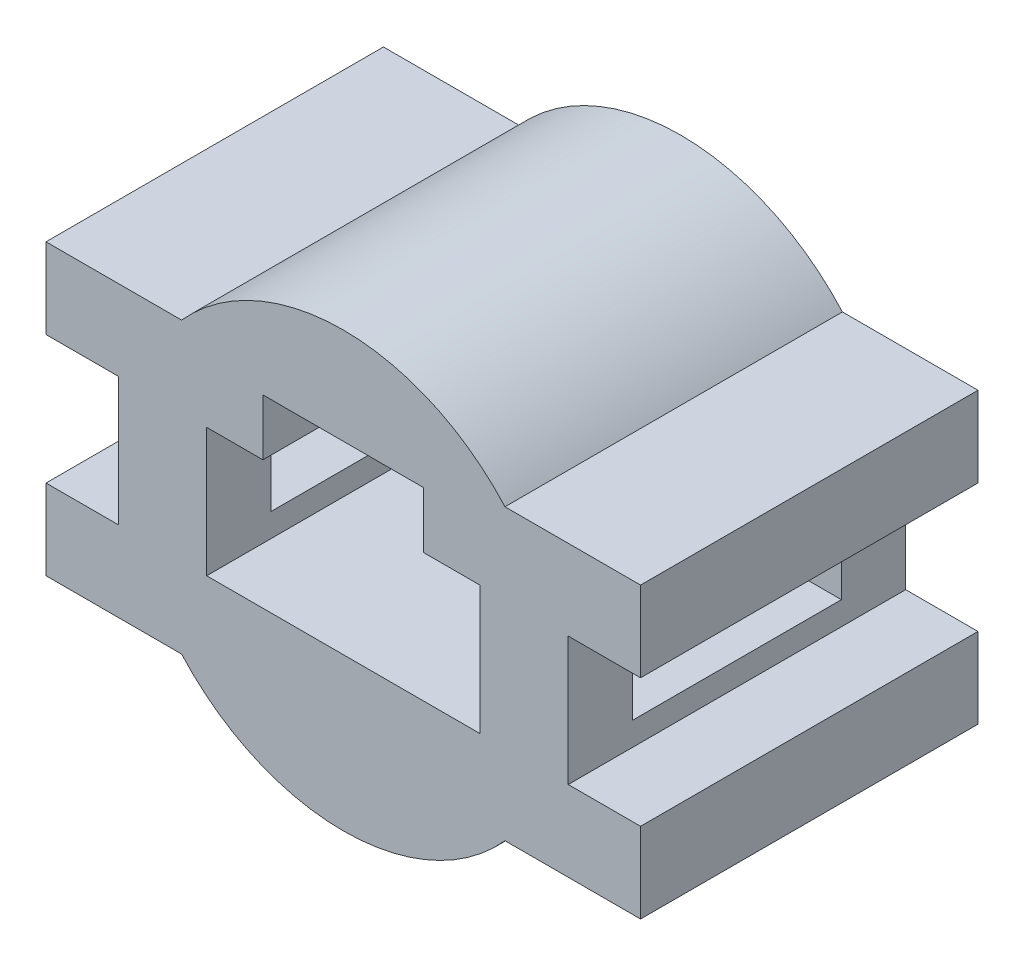
ISO-10303-21;
HEADER;
FILE_DESCRIPTION(('STEP AP214'),'2;1');
FILE_NAME('part.step','',(''),(''),'','','');
FILE_SCHEMA(('AUTOMOTIVE_DESIGN { 1 0 10303 214 1 1 1 1 }'));
ENDSEC;
DATA;
#1=APPLICATION_CONTEXT('core data for automotive mechanical design processes');
#2=APPLICATION_PROTOCOL_DEFINITION('international standard','automotive_design',2000,#1);
#3=PRODUCT_CONTEXT('',#1,'mechanical');
#4=PRODUCT('Part','Part','',(#3));
#5=PRODUCT_RELATED_PRODUCT_CATEGORY('part','',(#4));
#6=PRODUCT_DEFINITION_FORMATION('','',#4);
#7=PRODUCT_DEFINITION_CONTEXT('part definition',#1,'design');
#8=PRODUCT_DEFINITION('design','',#6,#7);
#9=PRODUCT_DEFINITION_SHAPE('','',#8);
#10=(LENGTH_UNIT() NAMED_UNIT(*) SI_UNIT(.MILLI.,.METRE.));
#11=(NAMED_UNIT(*) PLANE_ANGLE_UNIT() SI_UNIT($,.RADIAN.));
#12=(NAMED_UNIT(*) SI_UNIT($,.STERADIAN.) SOLID_ANGLE_UNIT());
#13=UNCERTAINTY_MEASURE_WITH_UNIT(LENGTH_MEASURE(1.E-05),#10,'distance_accuracy_value','');
#14=(GEOMETRIC_REPRESENTATION_CONTEXT(3) GLOBAL_UNCERTAINTY_ASSIGNED_CONTEXT((#13)) GLOBAL_UNIT_ASSIGNED_CONTEXT((#10,
#11,#12)) REPRESENTATION_CONTEXT('',''));
#15=CARTESIAN_POINT('',(0.,0.,0.));
#16=DIRECTION('',(0.,0.,1.));
#17=DIRECTION('',(1.,0.,0.));
#18=AXIS2_PLACEMENT_3D('',#15,#16,#17);
#19=CARTESIAN_POINT('',(0.,0.,-42.));
#20=DIRECTION('',(-1.,0.,0.));
#21=DIRECTION('',(0.,0.,1.));
#22=AXIS2_PLACEMENT_3D('',#19,#20,#21);
#23=PLANE('',#22);
#24=DIRECTION('',(0.,-1.,0.));
#25=VECTOR('',#24,1.);
#26=CARTESIAN_POINT('',(0.,0.,0.));
#27=LINE('',#26,#25);
#28=CARTESIAN_POINT('',(0.,0.,0.));
#29=VERTEX_POINT('',#28);
#30=CARTESIAN_POINT('',(0.,-10.,0.));
#31=VERTEX_POINT('',#30);
#32=EDGE_CURVE('E356',#29,#31,#27,.T.);
#33=ORIENTED_EDGE('',*,*,#32,.F.);
#34=DIRECTION('',(0.,0.,1.));
#35=VECTOR('',#34,1.);
#36=CARTESIAN_POINT('',(0.,0.,-42.));
#37=LINE('',#36,#35);
#38=CARTESIAN_POINT('',(0.,0.,-42.));
#39=VERTEX_POINT('',#38);
#40=EDGE_CURVE('E462',#39,#29,#37,.T.);
#41=ORIENTED_EDGE('',*,*,#40,.F.);
#42=DIRECTION('',(0.,-1.,0.));
#43=VECTOR('',#42,1.);
#44=CARTESIAN_POINT('',(0.,0.,-42.));
#45=LINE('',#44,#43);
#46=CARTESIAN_POINT('',(0.,-10.,-42.));
#47=VERTEX_POINT('',#46);
#48=EDGE_CURVE('E364',#39,#47,#45,.T.);
#49=ORIENTED_EDGE('',*,*,#48,.T.);
#50=DIRECTION('',(0.,0.,1.));
#51=VECTOR('',#50,1.);
#52=CARTESIAN_POINT('',(0.,-10.,-42.));
#53=LINE('',#52,#51);
#54=EDGE_CURVE('E412',#47,#31,#53,.T.);
#55=ORIENTED_EDGE('',*,*,#54,.T.);
#56=EDGE_LOOP('',(#33,#41,#49,#55));
#57=FACE_BOUND('',#56,.T.);
#58=ADVANCED_FACE('F39',(#57),#23,.T.);
#59=CARTESIAN_POINT('',(0.,0.,-42.));
#60=DIRECTION('',(0.,1.,0.));
#61=DIRECTION('',(0.,0.,1.));
#62=AXIS2_PLACEMENT_3D('',#59,#60,#61);
#63=PLANE('',#62);
#64=DIRECTION('',(-1.,0.,0.));
#65=VECTOR('',#64,1.);
#66=CARTESIAN_POINT('',(0.,0.,0.));
#67=LINE('',#66,#65);
#68=CARTESIAN_POINT('',(16.8753882025019,0.,0.));
#69=VERTEX_POINT('',#68);
#70=EDGE_CURVE('E369',#69,#29,#67,.T.);
#71=ORIENTED_EDGE('',*,*,#70,.F.);
#72=DIRECTION('',(0.,0.,1.));
#73=VECTOR('',#72,1.);
#74=CARTESIAN_POINT('',(16.8753882025019,0.,-42.));
#75=LINE('',#74,#73);
#76=CARTESIAN_POINT('',(16.8753882025019,0.,-42.));
#77=VERTEX_POINT('',#76);
#78=EDGE_CURVE('E461',#77,#69,#75,.T.);
#79=ORIENTED_EDGE('',*,*,#78,.F.);
#80=DIRECTION('',(-1.,0.,0.));
#81=VECTOR('',#80,1.);
#82=CARTESIAN_POINT('',(0.,0.,-42.));
#83=LINE('',#82,#81);
#84=EDGE_CURVE('E413',#77,#39,#83,.T.);
#85=ORIENTED_EDGE('',*,*,#84,.T.);
#86=ORIENTED_EDGE('',*,*,#40,.T.);
#87=EDGE_LOOP('',(#71,#79,#85,#86));
#88=FACE_BOUND('',#87,.T.);
#89=ADVANCED_FACE('F513',(#88),#63,.T.);
#90=CARTESIAN_POINT('',(37.,-18.,-42.));
#91=DIRECTION('',(0.,0.,1.));
#92=DIRECTION('',(1.,0.,0.));
#93=AXIS2_PLACEMENT_3D('',#90,#91,#92);
#94=CYLINDRICAL_SURFACE('',#93,27.);
#95=CARTESIAN_POINT('',(37.,-18.,0.));
#96=DIRECTION('',(0.,0.,1.));
#97=DIRECTION('',(1.,0.,0.));
#98=AXIS2_PLACEMENT_3D('',#95,#96,#97);
#99=CIRCLE('',#98,27.);
#100=CARTESIAN_POINT('',(57.1246117974981,0.,0.));
#101=VERTEX_POINT('',#100);
#102=EDGE_CURVE('E457',#101,#69,#99,.T.);
#103=ORIENTED_EDGE('',*,*,#102,.F.);
#104=DIRECTION('',(0.,0.,1.));
#105=VECTOR('',#104,1.);
#106=CARTESIAN_POINT('',(57.1246117974981,0.,-42.));
#107=LINE('',#106,#105);
#108=CARTESIAN_POINT('',(57.1246117974981,0.,-42.));
#109=VERTEX_POINT('',#108);
#110=EDGE_CURVE('E468',#109,#101,#107,.T.);
#111=ORIENTED_EDGE('',*,*,#110,.F.);
#112=CARTESIAN_POINT('',(37.,-18.,-42.));
#113=DIRECTION('',(0.,0.,1.));
#114=DIRECTION('',(1.,0.,0.));
#115=AXIS2_PLACEMENT_3D('',#112,#113,#114);
#116=CIRCLE('',#115,27.);
#117=EDGE_CURVE('E410',#109,#77,#116,.T.);
#118=ORIENTED_EDGE('',*,*,#117,.T.);
#119=ORIENTED_EDGE('',*,*,#78,.T.);
#120=EDGE_LOOP('',(#103,#111,#118,#119));
#121=FACE_BOUND('',#120,.T.);
#122=ADVANCED_FACE('F518',(#121),#94,.T.);
#123=CARTESIAN_POINT('',(57.1246117974981,0.,-42.));
#124=DIRECTION('',(0.,1.,0.));
#125=DIRECTION('',(0.,0.,1.));
#126=AXIS2_PLACEMENT_3D('',#123,#124,#125);
#127=PLANE('',#126);
#128=DIRECTION('',(-1.,0.,0.));
#129=VECTOR('',#128,1.);
#130=CARTESIAN_POINT('',(57.1246117974981,0.,0.));
#131=LINE('',#130,#129);
#132=CARTESIAN_POINT('',(74.,0.,0.));
#133=VERTEX_POINT('',#132);
#134=EDGE_CURVE('E451',#133,#101,#131,.T.);
#135=ORIENTED_EDGE('',*,*,#134,.F.);
#136=DIRECTION('',(0.,0.,1.));
#137=VECTOR('',#136,1.);
#138=CARTESIAN_POINT('',(74.,0.,-42.));
#139=LINE('',#138,#137);
#140=CARTESIAN_POINT('',(74.,0.,-42.));
#141=VERTEX_POINT('',#140);
#142=EDGE_CURVE('E466',#141,#133,#139,.T.);
#143=ORIENTED_EDGE('',*,*,#142,.F.);
#144=DIRECTION('',(-1.,0.,0.));
#145=VECTOR('',#144,1.);
#146=CARTESIAN_POINT('',(57.1246117974981,0.,-42.));
#147=LINE('',#146,#145);
#148=EDGE_CURVE('E403',#141,#109,#147,.T.);
#149=ORIENTED_EDGE('',*,*,#148,.T.);
#150=ORIENTED_EDGE('',*,*,#110,.T.);
#151=EDGE_LOOP('',(#135,#143,#149,#150));
#152=FACE_BOUND('',#151,.T.);
#153=ADVANCED_FACE('F582',(#152),#127,.T.);
#154=CARTESIAN_POINT('',(74.,0.,-42.));
#155=DIRECTION('',(1.,0.,0.));
#156=DIRECTION('',(0.,0.,-1.));
#157=AXIS2_PLACEMENT_3D('',#154,#155,#156);
#158=PLANE('',#157);
#159=DIRECTION('',(0.,1.,0.));
#160=VECTOR('',#159,1.);
#161=CARTESIAN_POINT('',(74.,0.,0.));
#162=LINE('',#161,#160);
#163=CARTESIAN_POINT('',(74.,-10.,0.));
#164=VERTEX_POINT('',#163);
#165=EDGE_CURVE('E448',#164,#133,#162,.T.);
#166=ORIENTED_EDGE('',*,*,#165,.F.);
#167=DIRECTION('',(0.,0.,1.));
#168=VECTOR('',#167,1.);
#169=CARTESIAN_POINT('',(74.,-10.,-42.));
#170=LINE('',#169,#168);
#171=CARTESIAN_POINT('',(74.,-10.,-42.));
#172=VERTEX_POINT('',#171);
#173=EDGE_CURVE('E469',#172,#164,#170,.T.);
#174=ORIENTED_EDGE('',*,*,#173,.F.);
#175=DIRECTION('',(0.,1.,0.));
#176=VECTOR('',#175,1.);
#177=CARTESIAN_POINT('',(74.,0.,-42.));
#178=LINE('',#177,#176);
#179=EDGE_CURVE('E405',#172,#141,#178,.T.);
#180=ORIENTED_EDGE('',*,*,#179,.T.);
#181=ORIENTED_EDGE('',*,*,#142,.T.);
#182=EDGE_LOOP('',(#166,#174,#180,#181));
#183=FACE_BOUND('',#182,.T.);
#184=ADVANCED_FACE('F577',(#183),#158,.T.);
#185=CARTESIAN_POINT('',(74.,-10.,-42.));
#186=DIRECTION('',(0.,-1.,0.));
#187=DIRECTION('',(0.,0.,-1.));
#188=AXIS2_PLACEMENT_3D('',#185,#186,#187);
#189=PLANE('',#188);
#190=DIRECTION('',(1.,0.,0.));
#191=VECTOR('',#190,1.);
#192=CARTESIAN_POINT('',(74.,-10.,0.));
#193=LINE('',#192,#191);
#194=CARTESIAN_POINT('',(65.,-10.,0.));
#195=VERTEX_POINT('',#194);
#196=EDGE_CURVE('E449',#195,#164,#193,.T.);
#197=ORIENTED_EDGE('',*,*,#196,.F.);
#198=DIRECTION('',(0.,0.,1.));
#199=VECTOR('',#198,1.);
#200=CARTESIAN_POINT('',(65.,-10.,-42.));
#201=LINE('',#200,#199);
#202=CARTESIAN_POINT('',(65.,-10.,-42.));
#203=VERTEX_POINT('',#202);
#204=EDGE_CURVE('E472',#203,#195,#201,.T.);
#205=ORIENTED_EDGE('',*,*,#204,.F.);
#206=DIRECTION('',(1.,0.,0.));
#207=VECTOR('',#206,1.);
#208=CARTESIAN_POINT('',(74.,-10.,-42.));
#209=LINE('',#208,#207);
#210=EDGE_CURVE('E397',#203,#172,#209,.T.);
#211=ORIENTED_EDGE('',*,*,#210,.T.);
#212=ORIENTED_EDGE('',*,*,#173,.T.);
#213=EDGE_LOOP('',(#197,#205,#211,#212));
#214=FACE_BOUND('',#213,.T.);
#215=ADVANCED_FACE('F573',(#214),#189,.T.);
#216=CARTESIAN_POINT('',(65.,-10.,-42.));
#217=DIRECTION('',(1.,0.,0.));
#218=DIRECTION('',(0.,0.,-1.));
#219=AXIS2_PLACEMENT_3D('',#216,#217,#218);
#220=PLANE('',#219);
#221=DIRECTION('',(0.,0.,1.));
#222=VECTOR('',#221,1.);
#223=CARTESIAN_POINT('',(65.,-13.075177639069,-42.));
#224=LINE('',#223,#222);
#225=CARTESIAN_POINT('',(65.,-13.075177639069,-34.));
#226=VERTEX_POINT('',#225);
#227=CARTESIAN_POINT('',(65.,-13.075177639069,-8.00000000000001));
#228=VERTEX_POINT('',#227);
#229=EDGE_CURVE('E298',#226,#228,#224,.T.);
#230=ORIENTED_EDGE('',*,*,#229,.F.);
#231=DIRECTION('',(0.,1.,0.));
#232=VECTOR('',#231,1.);
#233=CARTESIAN_POINT('',(65.,-10.,-34.));
#234=LINE('',#233,#232);
#235=CARTESIAN_POINT('',(65.,-23.075177639069,-34.));
#236=VERTEX_POINT('',#235);
#237=EDGE_CURVE('E283',#236,#226,#234,.T.);
#238=ORIENTED_EDGE('',*,*,#237,.F.);
#239=DIRECTION('',(0.,0.,-1.));
#240=VECTOR('',#239,1.);
#241=CARTESIAN_POINT('',(65.,-23.075177639069,-42.));
#242=LINE('',#241,#240);
#243=CARTESIAN_POINT('',(65.,-23.075177639069,-8.));
#244=VERTEX_POINT('',#243);
#245=EDGE_CURVE('E289',#244,#236,#242,.T.);
#246=ORIENTED_EDGE('',*,*,#245,.F.);
#247=DIRECTION('',(0.,-1.,0.));
#248=VECTOR('',#247,1.);
#249=CARTESIAN_POINT('',(65.,-9.99999999999999,-8.00000000000001));
#250=LINE('',#249,#248);
#251=EDGE_CURVE('E293',#228,#244,#250,.T.);
#252=ORIENTED_EDGE('',*,*,#251,.F.);
#253=EDGE_LOOP('',(#230,#238,#246,#252));
#254=FACE_BOUND('',#253,.T.);
#255=DIRECTION('',(0.,1.,0.));
#256=VECTOR('',#255,1.);
#257=CARTESIAN_POINT('',(65.,-10.,0.));
#258=LINE('',#257,#256);
#259=CARTESIAN_POINT('',(65.,-26.,0.));
#260=VERTEX_POINT('',#259);
#261=EDGE_CURVE('E441',#260,#195,#258,.T.);
#262=ORIENTED_EDGE('',*,*,#261,.F.);
#263=DIRECTION('',(0.,0.,1.));
#264=VECTOR('',#263,1.);
#265=CARTESIAN_POINT('',(65.,-26.,-42.));
#266=LINE('',#265,#264);
#267=CARTESIAN_POINT('',(65.,-26.,-42.));
#268=VERTEX_POINT('',#267);
#269=EDGE_CURVE('E475',#268,#260,#266,.T.);
#270=ORIENTED_EDGE('',*,*,#269,.F.);
#271=DIRECTION('',(0.,1.,0.));
#272=VECTOR('',#271,1.);
#273=CARTESIAN_POINT('',(65.,-10.,-42.));
#274=LINE('',#273,#272);
#275=EDGE_CURVE('E398',#268,#203,#274,.T.);
#276=ORIENTED_EDGE('',*,*,#275,.T.);
#277=ORIENTED_EDGE('',*,*,#204,.T.);
#278=EDGE_LOOP('',(#262,#270,#276,#277));
#279=FACE_BOUND('',#278,.T.);
#280=ADVANCED_FACE('F572',(#254,#279),#220,.T.);
#281=CARTESIAN_POINT('',(65.,-26.,-42.));
#282=DIRECTION('',(0.,1.,0.));
#283=DIRECTION('',(0.,0.,1.));
#284=AXIS2_PLACEMENT_3D('',#281,#282,#283);
#285=PLANE('',#284);
#286=DIRECTION('',(-1.,0.,0.));
#287=VECTOR('',#286,1.);
#288=CARTESIAN_POINT('',(65.,-26.,0.));
#289=LINE('',#288,#287);
#290=CARTESIAN_POINT('',(74.,-26.,0.));
#291=VERTEX_POINT('',#290);
#292=EDGE_CURVE('E442',#291,#260,#289,.T.);
#293=ORIENTED_EDGE('',*,*,#292,.F.);
#294=DIRECTION('',(0.,0.,1.));
#295=VECTOR('',#294,1.);
#296=CARTESIAN_POINT('',(74.,-26.,-42.));
#297=LINE('',#296,#295);
#298=CARTESIAN_POINT('',(74.,-26.,-42.));
#299=VERTEX_POINT('',#298);
#300=EDGE_CURVE('E478',#299,#291,#297,.T.);
#301=ORIENTED_EDGE('',*,*,#300,.F.);
#302=DIRECTION('',(-1.,0.,0.));
#303=VECTOR('',#302,1.);
#304=CARTESIAN_POINT('',(65.,-26.,-42.));
#305=LINE('',#304,#303);
#306=EDGE_CURVE('E395',#299,#268,#305,.T.);
#307=ORIENTED_EDGE('',*,*,#306,.T.);
#308=ORIENTED_EDGE('',*,*,#269,.T.);
#309=EDGE_LOOP('',(#293,#301,#307,#308));
#310=FACE_BOUND('',#309,.T.);
#311=ADVANCED_FACE('F570',(#310),#285,.T.);
#312=CARTESIAN_POINT('',(74.,-26.,-42.));
#313=DIRECTION('',(1.,0.,0.));
#314=DIRECTION('',(0.,1.,0.));
#315=AXIS2_PLACEMENT_3D('',#312,#313,#314);
#316=PLANE('',#315);
#317=DIRECTION('',(0.,1.,0.));
#318=VECTOR('',#317,1.);
#319=CARTESIAN_POINT('',(74.,-26.,0.));
#320=LINE('',#319,#318);
#321=CARTESIAN_POINT('',(74.,-36.,0.));
#322=VERTEX_POINT('',#321);
#323=EDGE_CURVE('E437',#322,#291,#320,.T.);
#324=ORIENTED_EDGE('',*,*,#323,.F.);
#325=DIRECTION('',(0.,0.,1.));
#326=VECTOR('',#325,1.);
#327=CARTESIAN_POINT('',(74.,-36.,-42.));
#328=LINE('',#327,#326);
#329=CARTESIAN_POINT('',(74.,-36.,-42.));
#330=VERTEX_POINT('',#329);
#331=EDGE_CURVE('E476',#330,#322,#328,.T.);
#332=ORIENTED_EDGE('',*,*,#331,.F.);
#333=DIRECTION('',(0.,1.,0.));
#334=VECTOR('',#333,1.);
#335=CARTESIAN_POINT('',(74.,-26.,-42.));
#336=LINE('',#335,#334);
#337=EDGE_CURVE('E388',#330,#299,#336,.T.);
#338=ORIENTED_EDGE('',*,*,#337,.T.);
#339=ORIENTED_EDGE('',*,*,#300,.T.);
#340=EDGE_LOOP('',(#324,#332,#338,#339));
#341=FACE_BOUND('',#340,.T.);
#342=ADVANCED_FACE('F561',(#341),#316,.T.);
#343=CARTESIAN_POINT('',(74.,-36.,-42.));
#344=DIRECTION('',(0.,-1.,0.));
#345=DIRECTION('',(0.,0.,-1.));
#346=AXIS2_PLACEMENT_3D('',#343,#344,#345);
#347=PLANE('',#346);
#348=DIRECTION('',(1.,0.,0.));
#349=VECTOR('',#348,1.);
#350=CARTESIAN_POINT('',(74.,-36.,0.));
#351=LINE('',#350,#349);
#352=CARTESIAN_POINT('',(57.1246117974981,-36.,0.));
#353=VERTEX_POINT('',#352);
#354=EDGE_CURVE('E434',#353,#322,#351,.T.);
#355=ORIENTED_EDGE('',*,*,#354,.F.);
#356=DIRECTION('',(0.,0.,1.));
#357=VECTOR('',#356,1.);
#358=CARTESIAN_POINT('',(57.1246117974981,-36.,-42.));
#359=LINE('',#358,#357);
#360=CARTESIAN_POINT('',(57.1246117974981,-36.,-42.));
#361=VERTEX_POINT('',#360);
#362=EDGE_CURVE('E477',#361,#353,#359,.T.);
#363=ORIENTED_EDGE('',*,*,#362,.F.);
#364=DIRECTION('',(1.,0.,0.));
#365=VECTOR('',#364,1.);
#366=CARTESIAN_POINT('',(74.,-36.,-42.));
#367=LINE('',#366,#365);
#368=EDGE_CURVE('E390',#361,#330,#367,.T.);
#369=ORIENTED_EDGE('',*,*,#368,.T.);
#370=ORIENTED_EDGE('',*,*,#331,.T.);
#371=EDGE_LOOP('',(#355,#363,#369,#370));
#372=FACE_BOUND('',#371,.T.);
#373=ADVANCED_FACE('F556',(#372),#347,.T.);
#374=CARTESIAN_POINT('',(37.,-18.,-42.));
#375=DIRECTION('',(0.,0.,1.));
#376=DIRECTION('',(1.,0.,0.));
#377=AXIS2_PLACEMENT_3D('',#374,#375,#376);
#378=CYLINDRICAL_SURFACE('',#377,27.);
#379=CARTESIAN_POINT('',(37.,-18.,0.));
#380=DIRECTION('',(0.,0.,1.));
#381=DIRECTION('',(1.,0.,0.));
#382=AXIS2_PLACEMENT_3D('',#379,#380,#381);
#383=CIRCLE('',#382,27.);
#384=CARTESIAN_POINT('',(16.8753882025019,-36.,0.));
#385=VERTEX_POINT('',#384);
#386=EDGE_CURVE('E435',#385,#353,#383,.T.);
#387=ORIENTED_EDGE('',*,*,#386,.F.);
#388=DIRECTION('',(0.,0.,1.));
#389=VECTOR('',#388,1.);
#390=CARTESIAN_POINT('',(16.8753882025019,-36.,-42.));
#391=LINE('',#390,#389);
#392=CARTESIAN_POINT('',(16.8753882025019,-36.,-42.));
#393=VERTEX_POINT('',#392);
#394=EDGE_CURVE('E485',#393,#385,#391,.T.);
#395=ORIENTED_EDGE('',*,*,#394,.F.);
#396=CARTESIAN_POINT('',(37.,-18.,-42.));
#397=DIRECTION('',(0.,0.,1.));
#398=DIRECTION('',(1.,0.,0.));
#399=AXIS2_PLACEMENT_3D('',#396,#397,#398);
#400=CIRCLE('',#399,27.);
#401=EDGE_CURVE('E383',#393,#361,#400,.T.);
#402=ORIENTED_EDGE('',*,*,#401,.T.);
#403=ORIENTED_EDGE('',*,*,#362,.T.);
#404=EDGE_LOOP('',(#387,#395,#402,#403));
#405=FACE_BOUND('',#404,.T.);
#406=ADVANCED_FACE('F553',(#405),#378,.T.);
#407=CARTESIAN_POINT('',(16.8753882025019,-36.,-42.));
#408=DIRECTION('',(0.,-1.,0.));
#409=DIRECTION('',(0.,0.,-1.));
#410=AXIS2_PLACEMENT_3D('',#407,#408,#409);
#411=PLANE('',#410);
#412=DIRECTION('',(1.,0.,0.));
#413=VECTOR('',#412,1.);
#414=CARTESIAN_POINT('',(16.8753882025019,-36.,0.));
#415=LINE('',#414,#413);
#416=CARTESIAN_POINT('',(0.,-36.,0.));
#417=VERTEX_POINT('',#416);
#418=EDGE_CURVE('E427',#417,#385,#415,.T.);
#419=ORIENTED_EDGE('',*,*,#418,.F.);
#420=DIRECTION('',(0.,0.,1.));
#421=VECTOR('',#420,1.);
#422=CARTESIAN_POINT('',(0.,-36.,-42.));
#423=LINE('',#422,#421);
#424=CARTESIAN_POINT('',(0.,-36.,-42.));
#425=VERTEX_POINT('',#424);
#426=EDGE_CURVE('E482',#425,#417,#423,.T.);
#427=ORIENTED_EDGE('',*,*,#426,.F.);
#428=DIRECTION('',(1.,0.,0.));
#429=VECTOR('',#428,1.);
#430=CARTESIAN_POINT('',(16.8753882025019,-36.,-42.));
#431=LINE('',#430,#429);
#432=EDGE_CURVE('E381',#425,#393,#431,.T.);
#433=ORIENTED_EDGE('',*,*,#432,.T.);
#434=ORIENTED_EDGE('',*,*,#394,.T.);
#435=EDGE_LOOP('',(#419,#427,#433,#434));
#436=FACE_BOUND('',#435,.T.);
#437=ADVANCED_FACE('F552',(#436),#411,.T.);
#438=CARTESIAN_POINT('',(0.,-26.,-42.));
#439=DIRECTION('',(-1.,0.,0.));
#440=DIRECTION('',(0.,-1.,0.));
#441=AXIS2_PLACEMENT_3D('',#438,#439,#440);
#442=PLANE('',#441);
#443=DIRECTION('',(0.,-1.,0.));
#444=VECTOR('',#443,1.);
#445=CARTESIAN_POINT('',(0.,-26.,0.));
#446=LINE('',#445,#444);
#447=CARTESIAN_POINT('',(0.,-26.,0.));
#448=VERTEX_POINT('',#447);
#449=EDGE_CURVE('E426',#448,#417,#446,.T.);
#450=ORIENTED_EDGE('',*,*,#449,.F.);
#451=DIRECTION('',(0.,0.,1.));
#452=VECTOR('',#451,1.);
#453=CARTESIAN_POINT('',(0.,-26.,-42.));
#454=LINE('',#453,#452);
#455=CARTESIAN_POINT('',(0.,-26.,-42.));
#456=VERTEX_POINT('',#455);
#457=EDGE_CURVE('E486',#456,#448,#454,.T.);
#458=ORIENTED_EDGE('',*,*,#457,.F.);
#459=DIRECTION('',(0.,-1.,0.));
#460=VECTOR('',#459,1.);
#461=CARTESIAN_POINT('',(0.,-26.,-42.));
#462=LINE('',#461,#460);
#463=EDGE_CURVE('E378',#456,#425,#462,.T.);
#464=ORIENTED_EDGE('',*,*,#463,.T.);
#465=ORIENTED_EDGE('',*,*,#426,.T.);
#466=EDGE_LOOP('',(#450,#458,#464,#465));
#467=FACE_BOUND('',#466,.T.);
#468=ADVANCED_FACE('F550',(#467),#442,.T.);
#469=CARTESIAN_POINT('',(8.99999999999999,-26.,-42.));
#470=DIRECTION('',(0.,1.,0.));
#471=DIRECTION('',(0.,0.,1.));
#472=AXIS2_PLACEMENT_3D('',#469,#470,#471);
#473=PLANE('',#472);
#474=DIRECTION('',(-1.,0.,0.));
#475=VECTOR('',#474,1.);
#476=CARTESIAN_POINT('',(8.99999999999999,-26.,0.));
#477=LINE('',#476,#475);
#478=CARTESIAN_POINT('',(8.99999999999999,-26.,0.));
#479=VERTEX_POINT('',#478);
#480=EDGE_CURVE('E421',#479,#448,#477,.T.);
#481=ORIENTED_EDGE('',*,*,#480,.F.);
#482=DIRECTION('',(0.,0.,1.));
#483=VECTOR('',#482,1.);
#484=CARTESIAN_POINT('',(8.99999999999999,-26.,-42.));
#485=LINE('',#484,#483);
#486=CARTESIAN_POINT('',(8.99999999999999,-26.,-42.));
#487=VERTEX_POINT('',#486);
#488=EDGE_CURVE('E488',#487,#479,#485,.T.);
#489=ORIENTED_EDGE('',*,*,#488,.F.);
#490=DIRECTION('',(-1.,0.,0.));
#491=VECTOR('',#490,1.);
#492=CARTESIAN_POINT('',(8.99999999999999,-26.,-42.));
#493=LINE('',#492,#491);
#494=EDGE_CURVE('E374',#487,#456,#493,.T.);
#495=ORIENTED_EDGE('',*,*,#494,.T.);
#496=ORIENTED_EDGE('',*,*,#457,.T.);
#497=EDGE_LOOP('',(#481,#489,#495,#496));
#498=FACE_BOUND('',#497,.T.);
#499=ADVANCED_FACE('F543',(#498),#473,.T.);
#500=CARTESIAN_POINT('',(8.99999999999999,-10.,-42.));
#501=DIRECTION('',(-1.,0.,0.));
#502=DIRECTION('',(0.,-1.,0.));
#503=AXIS2_PLACEMENT_3D('',#500,#501,#502);
#504=PLANE('',#503);
#505=DIRECTION('',(0.,0.,-1.));
#506=VECTOR('',#505,1.);
#507=CARTESIAN_POINT('',(8.99999999999999,-13.075177639069,-34.));
#508=LINE('',#507,#506);
#509=CARTESIAN_POINT('',(8.99999999999999,-13.075177639069,-8.00000000000001));
#510=VERTEX_POINT('',#509);
#511=CARTESIAN_POINT('',(8.99999999999999,-13.075177639069,-34.));
#512=VERTEX_POINT('',#511);
#513=EDGE_CURVE('E62',#510,#512,#508,.T.);
#514=ORIENTED_EDGE('',*,*,#513,.F.);
#515=DIRECTION('',(0.,1.,0.));
#516=VECTOR('',#515,1.);
#517=CARTESIAN_POINT('',(8.99999999999999,-13.075177639069,-8.00000000000001));
#518=LINE('',#517,#516);
#519=CARTESIAN_POINT('',(8.99999999999999,-23.075177639069,-8.));
#520=VERTEX_POINT('',#519);
#521=EDGE_CURVE('E269',#520,#510,#518,.T.);
#522=ORIENTED_EDGE('',*,*,#521,.F.);
#523=DIRECTION('',(0.,0.,1.));
#524=VECTOR('',#523,1.);
#525=CARTESIAN_POINT('',(8.99999999999999,-23.075177639069,-8.));
#526=LINE('',#525,#524);
#527=CARTESIAN_POINT('',(8.99999999999999,-23.075177639069,-34.));
#528=VERTEX_POINT('',#527);
#529=EDGE_CURVE('E251',#528,#520,#526,.T.);
#530=ORIENTED_EDGE('',*,*,#529,.F.);
#531=DIRECTION('',(0.,-1.,0.));
#532=VECTOR('',#531,1.);
#533=CARTESIAN_POINT('',(8.99999999999999,-23.075177639069,-34.));
#534=LINE('',#533,#532);
#535=EDGE_CURVE('E265',#512,#528,#534,.T.);
#536=ORIENTED_EDGE('',*,*,#535,.F.);
#537=EDGE_LOOP('',(#514,#522,#530,#536));
#538=FACE_BOUND('',#537,.T.);
#539=DIRECTION('',(0.,-1.,0.));
#540=VECTOR('',#539,1.);
#541=CARTESIAN_POINT('',(8.99999999999999,-10.,0.));
#542=LINE('',#541,#540);
#543=CARTESIAN_POINT('',(8.99999999999999,-10.,0.));
#544=VERTEX_POINT('',#543);
#545=EDGE_CURVE('E419',#544,#479,#542,.T.);
#546=ORIENTED_EDGE('',*,*,#545,.F.);
#547=DIRECTION('',(0.,0.,1.));
#548=VECTOR('',#547,1.);
#549=CARTESIAN_POINT('',(8.99999999999999,-10.,-42.));
#550=LINE('',#549,#548);
#551=CARTESIAN_POINT('',(8.99999999999999,-10.,-42.));
#552=VERTEX_POINT('',#551);
#553=EDGE_CURVE('E489',#552,#544,#550,.T.);
#554=ORIENTED_EDGE('',*,*,#553,.F.);
#555=DIRECTION('',(0.,-1.,0.));
#556=VECTOR('',#555,1.);
#557=CARTESIAN_POINT('',(8.99999999999999,-10.,-42.));
#558=LINE('',#557,#556);
#559=EDGE_CURVE('E375',#552,#487,#558,.T.);
#560=ORIENTED_EDGE('',*,*,#559,.T.);
#561=ORIENTED_EDGE('',*,*,#488,.T.);
#562=EDGE_LOOP('',(#546,#554,#560,#561));
#563=FACE_BOUND('',#562,.T.);
#564=ADVANCED_FACE('F270',(#538,#563),#504,.T.);
#565=CARTESIAN_POINT('',(0.,-10.,-42.));
#566=DIRECTION('',(0.,-1.,0.));
#567=DIRECTION('',(0.,0.,-1.));
#568=AXIS2_PLACEMENT_3D('',#565,#566,#567);
#569=PLANE('',#568);
#570=DIRECTION('',(1.,0.,0.));
#571=VECTOR('',#570,1.);
#572=CARTESIAN_POINT('',(0.,-10.,0.));
#573=LINE('',#572,#571);
#574=EDGE_CURVE('E417',#31,#544,#573,.T.);
#575=ORIENTED_EDGE('',*,*,#574,.F.);
#576=ORIENTED_EDGE('',*,*,#54,.F.);
#577=DIRECTION('',(1.,0.,0.));
#578=VECTOR('',#577,1.);
#579=CARTESIAN_POINT('',(0.,-10.,-42.));
#580=LINE('',#579,#578);
#581=EDGE_CURVE('E366',#47,#552,#580,.T.);
#582=ORIENTED_EDGE('',*,*,#581,.T.);
#583=ORIENTED_EDGE('',*,*,#553,.T.);
#584=EDGE_LOOP('',(#575,#576,#582,#583));
#585=FACE_BOUND('',#584,.T.);
#586=ADVANCED_FACE('F537',(#585),#569,.T.);
#587=CARTESIAN_POINT('',(37.,-18.,-42.));
#588=DIRECTION('',(0.,0.,1.));
#589=DIRECTION('',(1.,0.,0.));
#590=AXIS2_PLACEMENT_3D('',#587,#588,#589);
#591=PLANE('',#590);
#592=DIRECTION('',(0.,1.,0.));
#593=VECTOR('',#592,1.);
#594=CARTESIAN_POINT('',(54.,-10.,-42.));
#595=LINE('',#594,#593);
#596=CARTESIAN_POINT('',(54.,-26.,-42.));
#597=VERTEX_POINT('',#596);
#598=CARTESIAN_POINT('',(54.,-10.,-42.));
#599=VERTEX_POINT('',#598);
#600=EDGE_CURVE('E343',#597,#599,#595,.T.);
#601=ORIENTED_EDGE('',*,*,#600,.T.);
#602=DIRECTION('',(-1.,0.,0.));
#603=VECTOR('',#602,1.);
#604=CARTESIAN_POINT('',(27.,-10.,-42.));
#605=LINE('',#604,#603);
#606=CARTESIAN_POINT('',(20.,-10.,-42.));
#607=VERTEX_POINT('',#606);
#608=EDGE_CURVE('E332',#599,#607,#605,.T.);
#609=ORIENTED_EDGE('',*,*,#608,.T.);
#610=DIRECTION('',(0.,-1.,0.));
#611=VECTOR('',#610,1.);
#612=CARTESIAN_POINT('',(20.,-26.,-42.));
#613=LINE('',#612,#611);
#614=CARTESIAN_POINT('',(20.,-26.,-42.));
#615=VERTEX_POINT('',#614);
#616=EDGE_CURVE('E331',#607,#615,#613,.T.);
#617=ORIENTED_EDGE('',*,*,#616,.T.);
#618=DIRECTION('',(1.,0.,0.));
#619=VECTOR('',#618,1.);
#620=CARTESIAN_POINT('',(54.,-26.,-42.));
#621=LINE('',#620,#619);
#622=EDGE_CURVE('E340',#615,#597,#621,.T.);
#623=ORIENTED_EDGE('',*,*,#622,.T.);
#624=EDGE_LOOP('',(#601,#609,#617,#623));
#625=FACE_BOUND('',#624,.T.);
#626=ORIENTED_EDGE('',*,*,#48,.F.);
#627=ORIENTED_EDGE('',*,*,#84,.F.);
#628=ORIENTED_EDGE('',*,*,#117,.F.);
#629=ORIENTED_EDGE('',*,*,#148,.F.);
#630=ORIENTED_EDGE('',*,*,#179,.F.);
#631=ORIENTED_EDGE('',*,*,#210,.F.);
#632=ORIENTED_EDGE('',*,*,#275,.F.);
#633=ORIENTED_EDGE('',*,*,#306,.F.);
#634=ORIENTED_EDGE('',*,*,#337,.F.);
#635=ORIENTED_EDGE('',*,*,#368,.F.);
#636=ORIENTED_EDGE('',*,*,#401,.F.);
#637=ORIENTED_EDGE('',*,*,#432,.F.);
#638=ORIENTED_EDGE('',*,*,#463,.F.);
#639=ORIENTED_EDGE('',*,*,#494,.F.);
#640=ORIENTED_EDGE('',*,*,#559,.F.);
#641=ORIENTED_EDGE('',*,*,#581,.F.);
#642=EDGE_LOOP('',(#626,#627,#628,#629,#630,#631,#632,#633,#634,#635,#636,#637,#638,#639,#640,#641));
#643=FACE_BOUND('',#642,.T.);
#644=ADVANCED_FACE('F531',(#625,#643),#591,.F.);
#645=CARTESIAN_POINT('',(37.,-18.,0.));
#646=DIRECTION('',(0.,0.,1.));
#647=DIRECTION('',(1.,0.,0.));
#648=AXIS2_PLACEMENT_3D('',#645,#646,#647);
#649=PLANE('',#648);
#650=DIRECTION('',(0.,-1.,0.));
#651=VECTOR('',#650,1.);
#652=CARTESIAN_POINT('',(27.,-10.,0.));
#653=LINE('',#652,#651);
#654=CARTESIAN_POINT('',(27.,-3.00000000000001,0.));
#655=VERTEX_POINT('',#654);
#656=CARTESIAN_POINT('',(27.,-10.,0.));
#657=VERTEX_POINT('',#656);
#658=EDGE_CURVE('E307',#655,#657,#653,.T.);
#659=ORIENTED_EDGE('',*,*,#658,.F.);
#660=DIRECTION('',(-1.,0.,0.));
#661=VECTOR('',#660,1.);
#662=CARTESIAN_POINT('',(27.,-3.00000000000001,0.));
#663=LINE('',#662,#661);
#664=CARTESIAN_POINT('',(47.,-3.00000000000001,0.));
#665=VERTEX_POINT('',#664);
#666=EDGE_CURVE('E318',#665,#655,#663,.T.);
#667=ORIENTED_EDGE('',*,*,#666,.F.);
#668=DIRECTION('',(0.,1.,0.));
#669=VECTOR('',#668,1.);
#670=CARTESIAN_POINT('',(47.,-3.00000000000001,0.));
#671=LINE('',#670,#669);
#672=CARTESIAN_POINT('',(47.,-10.,0.));
#673=VERTEX_POINT('',#672);
#674=EDGE_CURVE('E305',#673,#665,#671,.T.);
#675=ORIENTED_EDGE('',*,*,#674,.F.);
#676=DIRECTION('',(-1.,0.,0.));
#677=VECTOR('',#676,1.);
#678=CARTESIAN_POINT('',(47.,-10.,0.));
#679=LINE('',#678,#677);
#680=CARTESIAN_POINT('',(54.,-10.,0.));
#681=VERTEX_POINT('',#680);
#682=EDGE_CURVE('E333',#681,#673,#679,.T.);
#683=ORIENTED_EDGE('',*,*,#682,.F.);
#684=DIRECTION('',(0.,1.,0.));
#685=VECTOR('',#684,1.);
#686=CARTESIAN_POINT('',(54.,-10.,0.));
#687=LINE('',#686,#685);
#688=CARTESIAN_POINT('',(54.,-26.,0.));
#689=VERTEX_POINT('',#688);
#690=EDGE_CURVE('E348',#689,#681,#687,.T.);
#691=ORIENTED_EDGE('',*,*,#690,.F.);
#692=DIRECTION('',(1.,0.,0.));
#693=VECTOR('',#692,1.);
#694=CARTESIAN_POINT('',(54.,-26.,0.));
#695=LINE('',#694,#693);
#696=CARTESIAN_POINT('',(20.,-26.,0.));
#697=VERTEX_POINT('',#696);
#698=EDGE_CURVE('E350',#697,#689,#695,.T.);
#699=ORIENTED_EDGE('',*,*,#698,.F.);
#700=DIRECTION('',(0.,-1.,0.));
#701=VECTOR('',#700,1.);
#702=CARTESIAN_POINT('',(20.,-26.,0.));
#703=LINE('',#702,#701);
#704=CARTESIAN_POINT('',(20.,-10.,0.));
#705=VERTEX_POINT('',#704);
#706=EDGE_CURVE('E324',#705,#697,#703,.T.);
#707=ORIENTED_EDGE('',*,*,#706,.F.);
#708=EDGE_CURVE('E355',#657,#705,#679,.T.);
#709=ORIENTED_EDGE('',*,*,#708,.F.);
#710=EDGE_LOOP('',(#659,#667,#675,#683,#691,#699,#707,#709));
#711=FACE_BOUND('',#710,.T.);
#712=ORIENTED_EDGE('',*,*,#32,.T.);
#713=ORIENTED_EDGE('',*,*,#574,.T.);
#714=ORIENTED_EDGE('',*,*,#545,.T.);
#715=ORIENTED_EDGE('',*,*,#480,.T.);
#716=ORIENTED_EDGE('',*,*,#449,.T.);
#717=ORIENTED_EDGE('',*,*,#418,.T.);
#718=ORIENTED_EDGE('',*,*,#386,.T.);
#719=ORIENTED_EDGE('',*,*,#354,.T.);
#720=ORIENTED_EDGE('',*,*,#323,.T.);
#721=ORIENTED_EDGE('',*,*,#292,.T.);
#722=ORIENTED_EDGE('',*,*,#261,.T.);
#723=ORIENTED_EDGE('',*,*,#196,.T.);
#724=ORIENTED_EDGE('',*,*,#165,.T.);
#725=ORIENTED_EDGE('',*,*,#134,.T.);
#726=ORIENTED_EDGE('',*,*,#102,.T.);
#727=ORIENTED_EDGE('',*,*,#70,.T.);
#728=EDGE_LOOP('',(#712,#713,#714,#715,#716,#717,#718,#719,#720,#721,#722,#723,#724,#725,#726,#727));
#729=FACE_BOUND('',#728,.T.);
#730=ADVANCED_FACE('F526',(#711,#729),#649,.T.);
#731=CARTESIAN_POINT('',(47.,-10.,-42.));
#732=DIRECTION('',(0.,1.,0.));
#733=DIRECTION('',(-1.,0.,0.));
#734=AXIS2_PLACEMENT_3D('',#731,#732,#733);
#735=PLANE('',#734);
#736=DIRECTION('',(1.,0.,0.));
#737=VECTOR('',#736,1.);
#738=CARTESIAN_POINT('',(27.,-10.,-10.));
#739=LINE('',#738,#737);
#740=CARTESIAN_POINT('',(27.,-9.99999999999999,-10.));
#741=VERTEX_POINT('',#740);
#742=CARTESIAN_POINT('',(47.,-10.,-10.));
#743=VERTEX_POINT('',#742);
#744=EDGE_CURVE('E301',#741,#743,#739,.T.);
#745=ORIENTED_EDGE('',*,*,#744,.F.);
#746=DIRECTION('',(0.,0.,1.));
#747=VECTOR('',#746,1.);
#748=CARTESIAN_POINT('',(27.,-10.,-10.));
#749=LINE('',#748,#747);
#750=EDGE_CURVE('E325',#741,#657,#749,.T.);
#751=ORIENTED_EDGE('',*,*,#750,.T.);
#752=ORIENTED_EDGE('',*,*,#708,.T.);
#753=DIRECTION('',(0.,0.,1.));
#754=VECTOR('',#753,1.);
#755=CARTESIAN_POINT('',(20.,-10.,-42.));
#756=LINE('',#755,#754);
#757=EDGE_CURVE('E342',#607,#705,#756,.T.);
#758=ORIENTED_EDGE('',*,*,#757,.F.);
#759=ORIENTED_EDGE('',*,*,#608,.F.);
#760=DIRECTION('',(0.,0.,1.));
#761=VECTOR('',#760,1.);
#762=CARTESIAN_POINT('',(54.,-10.,-42.));
#763=LINE('',#762,#761);
#764=EDGE_CURVE('E358',#599,#681,#763,.T.);
#765=ORIENTED_EDGE('',*,*,#764,.T.);
#766=ORIENTED_EDGE('',*,*,#682,.T.);
#767=DIRECTION('',(0.,0.,1.));
#768=VECTOR('',#767,1.);
#769=CARTESIAN_POINT('',(47.,-10.,-10.));
#770=LINE('',#769,#768);
#771=EDGE_CURVE('E312',#743,#673,#770,.T.);
#772=ORIENTED_EDGE('',*,*,#771,.F.);
#773=EDGE_LOOP('',(#745,#751,#752,#758,#759,#765,#766,#772));
#774=FACE_BOUND('',#773,.T.);
#775=ADVANCED_FACE('F624',(#774),#735,.F.);
#776=CARTESIAN_POINT('',(54.,-10.,-42.));
#777=DIRECTION('',(1.,0.,0.));
#778=DIRECTION('',(0.,0.,-1.));
#779=AXIS2_PLACEMENT_3D('',#776,#777,#778);
#780=PLANE('',#779);
#781=DIRECTION('',(0.,1.,0.));
#782=VECTOR('',#781,1.);
#783=CARTESIAN_POINT('',(54.,-10.,-34.));
#784=LINE('',#783,#782);
#785=CARTESIAN_POINT('',(54.,-23.075177639069,-34.));
#786=VERTEX_POINT('',#785);
#787=CARTESIAN_POINT('',(54.,-13.075177639069,-34.));
#788=VERTEX_POINT('',#787);
#789=EDGE_CURVE('E284',#786,#788,#784,.T.);
#790=ORIENTED_EDGE('',*,*,#789,.T.);
#791=DIRECTION('',(0.,0.,1.));
#792=VECTOR('',#791,1.);
#793=CARTESIAN_POINT('',(54.,-13.075177639069,-42.));
#794=LINE('',#793,#792);
#795=CARTESIAN_POINT('',(54.,-13.075177639069,-8.00000000000001));
#796=VERTEX_POINT('',#795);
#797=EDGE_CURVE('E299',#788,#796,#794,.T.);
#798=ORIENTED_EDGE('',*,*,#797,.T.);
#799=DIRECTION('',(0.,-1.,0.));
#800=VECTOR('',#799,1.);
#801=CARTESIAN_POINT('',(54.,-9.99999999999999,-8.00000000000001));
#802=LINE('',#801,#800);
#803=CARTESIAN_POINT('',(54.,-23.075177639069,-8.));
#804=VERTEX_POINT('',#803);
#805=EDGE_CURVE('E295',#796,#804,#802,.T.);
#806=ORIENTED_EDGE('',*,*,#805,.T.);
#807=DIRECTION('',(0.,0.,-1.));
#808=VECTOR('',#807,1.);
#809=CARTESIAN_POINT('',(54.,-23.075177639069,-42.));
#810=LINE('',#809,#808);
#811=EDGE_CURVE('E290',#804,#786,#810,.T.);
#812=ORIENTED_EDGE('',*,*,#811,.T.);
#813=EDGE_LOOP('',(#790,#798,#806,#812));
#814=FACE_BOUND('',#813,.T.);
#815=ORIENTED_EDGE('',*,*,#690,.T.);
#816=ORIENTED_EDGE('',*,*,#764,.F.);
#817=ORIENTED_EDGE('',*,*,#600,.F.);
#818=DIRECTION('',(0.,0.,1.));
#819=VECTOR('',#818,1.);
#820=CARTESIAN_POINT('',(54.,-26.,-42.));
#821=LINE('',#820,#819);
#822=EDGE_CURVE('E357',#597,#689,#821,.T.);
#823=ORIENTED_EDGE('',*,*,#822,.T.);
#824=EDGE_LOOP('',(#815,#816,#817,#823));
#825=FACE_BOUND('',#824,.T.);
#826=ADVANCED_FACE('F635',(#814,#825),#780,.F.);
#827=CARTESIAN_POINT('',(54.,-26.,-42.));
#828=DIRECTION('',(0.,-1.,0.));
#829=DIRECTION('',(0.,0.,-1.));
#830=AXIS2_PLACEMENT_3D('',#827,#828,#829);
#831=PLANE('',#830);
#832=ORIENTED_EDGE('',*,*,#698,.T.);
#833=ORIENTED_EDGE('',*,*,#822,.F.);
#834=ORIENTED_EDGE('',*,*,#622,.F.);
#835=DIRECTION('',(0.,0.,1.));
#836=VECTOR('',#835,1.);
#837=CARTESIAN_POINT('',(20.,-26.,-42.));
#838=LINE('',#837,#836);
#839=EDGE_CURVE('E363',#615,#697,#838,.T.);
#840=ORIENTED_EDGE('',*,*,#839,.T.);
#841=EDGE_LOOP('',(#832,#833,#834,#840));
#842=FACE_BOUND('',#841,.T.);
#843=ADVANCED_FACE('F628',(#842),#831,.F.);
#844=CARTESIAN_POINT('',(20.,-26.,-42.));
#845=DIRECTION('',(-1.,0.,0.));
#846=DIRECTION('',(0.,0.,1.));
#847=AXIS2_PLACEMENT_3D('',#844,#845,#846);
#848=PLANE('',#847);
#849=DIRECTION('',(0.,1.,0.));
#850=VECTOR('',#849,1.);
#851=CARTESIAN_POINT('',(20.,-26.,-8.));
#852=LINE('',#851,#850);
#853=CARTESIAN_POINT('',(20.,-23.075177639069,-8.));
#854=VERTEX_POINT('',#853);
#855=CARTESIAN_POINT('',(20.,-13.075177639069,-8.00000000000001));
#856=VERTEX_POINT('',#855);
#857=EDGE_CURVE('E46',#854,#856,#852,.T.);
#858=ORIENTED_EDGE('',*,*,#857,.T.);
#859=DIRECTION('',(0.,0.,-1.));
#860=VECTOR('',#859,1.);
#861=CARTESIAN_POINT('',(20.,-13.075177639069,-42.));
#862=LINE('',#861,#860);
#863=CARTESIAN_POINT('',(20.,-13.075177639069,-34.));
#864=VERTEX_POINT('',#863);
#865=EDGE_CURVE('E11',#856,#864,#862,.T.);
#866=ORIENTED_EDGE('',*,*,#865,.T.);
#867=DIRECTION('',(0.,-1.,0.));
#868=VECTOR('',#867,1.);
#869=CARTESIAN_POINT('',(20.,-26.,-34.));
#870=LINE('',#869,#868);
#871=CARTESIAN_POINT('',(20.,-23.075177639069,-34.));
#872=VERTEX_POINT('',#871);
#873=EDGE_CURVE('E465',#864,#872,#870,.T.);
#874=ORIENTED_EDGE('',*,*,#873,.T.);
#875=DIRECTION('',(0.,0.,1.));
#876=VECTOR('',#875,1.);
#877=CARTESIAN_POINT('',(20.,-23.075177639069,-42.));
#878=LINE('',#877,#876);
#879=EDGE_CURVE('E258',#872,#854,#878,.T.);
#880=ORIENTED_EDGE('',*,*,#879,.T.);
#881=EDGE_LOOP('',(#858,#866,#874,#880));
#882=FACE_BOUND('',#881,.T.);
#883=ORIENTED_EDGE('',*,*,#706,.T.);
#884=ORIENTED_EDGE('',*,*,#839,.F.);
#885=ORIENTED_EDGE('',*,*,#616,.F.);
#886=ORIENTED_EDGE('',*,*,#757,.T.);
#887=EDGE_LOOP('',(#883,#884,#885,#886));
#888=FACE_BOUND('',#887,.T.);
#889=ADVANCED_FACE('F497',(#882,#888),#848,.F.);
#890=CARTESIAN_POINT('',(27.,-10.,-10.));
#891=DIRECTION('',(-1.,0.,0.));
#892=DIRECTION('',(0.,0.,1.));
#893=AXIS2_PLACEMENT_3D('',#890,#891,#892);
#894=PLANE('',#893);
#895=ORIENTED_EDGE('',*,*,#658,.T.);
#896=ORIENTED_EDGE('',*,*,#750,.F.);
#897=DIRECTION('',(0.,-1.,0.));
#898=VECTOR('',#897,1.);
#899=CARTESIAN_POINT('',(27.,-10.,-10.));
#900=LINE('',#899,#898);
#901=CARTESIAN_POINT('',(27.,-3.00000000000001,-10.));
#902=VERTEX_POINT('',#901);
#903=EDGE_CURVE('E311',#902,#741,#900,.T.);
#904=ORIENTED_EDGE('',*,*,#903,.F.);
#905=DIRECTION('',(0.,0.,1.));
#906=VECTOR('',#905,1.);
#907=CARTESIAN_POINT('',(27.,-3.00000000000001,-10.));
#908=LINE('',#907,#906);
#909=EDGE_CURVE('E326',#902,#655,#908,.T.);
#910=ORIENTED_EDGE('',*,*,#909,.T.);
#911=EDGE_LOOP('',(#895,#896,#904,#910));
#912=FACE_BOUND('',#911,.T.);
#913=ADVANCED_FACE('F626',(#912),#894,.F.);
#914=CARTESIAN_POINT('',(27.,-3.00000000000001,-10.));
#915=DIRECTION('',(0.,1.,0.));
#916=DIRECTION('',(0.,0.,1.));
#917=AXIS2_PLACEMENT_3D('',#914,#915,#916);
#918=PLANE('',#917);
#919=ORIENTED_EDGE('',*,*,#666,.T.);
#920=ORIENTED_EDGE('',*,*,#909,.F.);
#921=DIRECTION('',(-1.,0.,0.));
#922=VECTOR('',#921,1.);
#923=CARTESIAN_POINT('',(27.,-3.00000000000001,-10.));
#924=LINE('',#923,#922);
#925=CARTESIAN_POINT('',(47.,-3.00000000000001,-10.));
#926=VERTEX_POINT('',#925);
#927=EDGE_CURVE('E309',#926,#902,#924,.T.);
#928=ORIENTED_EDGE('',*,*,#927,.F.);
#929=DIRECTION('',(0.,0.,1.));
#930=VECTOR('',#929,1.);
#931=CARTESIAN_POINT('',(47.,-3.00000000000001,-10.));
#932=LINE('',#931,#930);
#933=EDGE_CURVE('E327',#926,#665,#932,.T.);
#934=ORIENTED_EDGE('',*,*,#933,.T.);
#935=EDGE_LOOP('',(#919,#920,#928,#934));
#936=FACE_BOUND('',#935,.T.);
#937=ADVANCED_FACE('F644',(#936),#918,.F.);
#938=CARTESIAN_POINT('',(47.,-3.00000000000001,-10.));
#939=DIRECTION('',(1.,0.,0.));
#940=DIRECTION('',(0.,0.,-1.));
#941=AXIS2_PLACEMENT_3D('',#938,#939,#940);
#942=PLANE('',#941);
#943=ORIENTED_EDGE('',*,*,#674,.T.);
#944=ORIENTED_EDGE('',*,*,#933,.F.);
#945=DIRECTION('',(0.,1.,0.));
#946=VECTOR('',#945,1.);
#947=CARTESIAN_POINT('',(47.,-3.00000000000001,-10.));
#948=LINE('',#947,#946);
#949=EDGE_CURVE('E308',#743,#926,#948,.T.);
#950=ORIENTED_EDGE('',*,*,#949,.F.);
#951=ORIENTED_EDGE('',*,*,#771,.T.);
#952=EDGE_LOOP('',(#943,#944,#950,#951));
#953=FACE_BOUND('',#952,.T.);
#954=ADVANCED_FACE('F639',(#953),#942,.F.);
#955=CARTESIAN_POINT('',(0.,0.,-10.));
#956=DIRECTION('',(0.,0.,-1.));
#957=DIRECTION('',(-1.,0.,0.));
#958=AXIS2_PLACEMENT_3D('',#955,#956,#957);
#959=PLANE('',#958);
#960=ORIENTED_EDGE('',*,*,#744,.T.);
#961=ORIENTED_EDGE('',*,*,#949,.T.);
#962=ORIENTED_EDGE('',*,*,#927,.T.);
#963=ORIENTED_EDGE('',*,*,#903,.T.);
#964=EDGE_LOOP('',(#960,#961,#962,#963));
#965=FACE_BOUND('',#964,.T.);
#966=ADVANCED_FACE('F641',(#965),#959,.F.);
#967=CARTESIAN_POINT('',(74.,-23.075177639069,-34.));
#968=DIRECTION('',(0.,0.,-1.));
#969=DIRECTION('',(-1.,0.,0.));
#970=AXIS2_PLACEMENT_3D('',#967,#968,#969);
#971=PLANE('',#970);
#972=DIRECTION('',(-1.,0.,0.));
#973=VECTOR('',#972,1.);
#974=CARTESIAN_POINT('',(74.,-13.075177639069,-34.));
#975=LINE('',#974,#973);
#976=EDGE_CURVE('E262',#864,#512,#975,.T.);
#977=ORIENTED_EDGE('',*,*,#976,.T.);
#978=ORIENTED_EDGE('',*,*,#535,.T.);
#979=DIRECTION('',(-1.,0.,0.));
#980=VECTOR('',#979,1.);
#981=CARTESIAN_POINT('',(74.,-23.075177639069,-34.));
#982=LINE('',#981,#980);
#983=EDGE_CURVE('E246',#872,#528,#982,.T.);
#984=ORIENTED_EDGE('',*,*,#983,.F.);
#985=ORIENTED_EDGE('',*,*,#873,.F.);
#986=EDGE_LOOP('',(#977,#978,#984,#985));
#987=FACE_BOUND('',#986,.T.);
#988=ADVANCED_FACE('F263',(#987),#971,.F.);
#989=CARTESIAN_POINT('',(74.,-23.075177639069,-8.));
#990=DIRECTION('',(0.,-1.,0.));
#991=DIRECTION('',(1.,0.,0.));
#992=AXIS2_PLACEMENT_3D('',#989,#990,#991);
#993=PLANE('',#992);
#994=ORIENTED_EDGE('',*,*,#983,.T.);
#995=ORIENTED_EDGE('',*,*,#529,.T.);
#996=DIRECTION('',(-1.,0.,0.));
#997=VECTOR('',#996,1.);
#998=CARTESIAN_POINT('',(74.,-23.075177639069,-8.));
#999=LINE('',#998,#997);
#1000=EDGE_CURVE('E276',#854,#520,#999,.T.);
#1001=ORIENTED_EDGE('',*,*,#1000,.F.);
#1002=ORIENTED_EDGE('',*,*,#879,.F.);
#1003=EDGE_LOOP('',(#994,#995,#1001,#1002));
#1004=FACE_BOUND('',#1003,.T.);
#1005=ADVANCED_FACE('F249',(#1004),#993,.F.);
#1006=CARTESIAN_POINT('',(74.,-13.075177639069,-8.00000000000001));
#1007=DIRECTION('',(0.,0.,1.));
#1008=DIRECTION('',(0.,-1.,0.));
#1009=AXIS2_PLACEMENT_3D('',#1006,#1007,#1008);
#1010=PLANE('',#1009);
#1011=ORIENTED_EDGE('',*,*,#1000,.T.);
#1012=ORIENTED_EDGE('',*,*,#521,.T.);
#1013=DIRECTION('',(-1.,0.,0.));
#1014=VECTOR('',#1013,1.);
#1015=CARTESIAN_POINT('',(74.,-13.075177639069,-8.00000000000001));
#1016=LINE('',#1015,#1014);
#1017=EDGE_CURVE('E274',#856,#510,#1016,.T.);
#1018=ORIENTED_EDGE('',*,*,#1017,.F.);
#1019=ORIENTED_EDGE('',*,*,#857,.F.);
#1020=EDGE_LOOP('',(#1011,#1012,#1018,#1019));
#1021=FACE_BOUND('',#1020,.T.);
#1022=ADVANCED_FACE('F498',(#1021),#1010,.F.);
#1023=CARTESIAN_POINT('',(74.,-13.075177639069,-34.));
#1024=DIRECTION('',(0.,1.,0.));
#1025=DIRECTION('',(-1.,0.,0.));
#1026=AXIS2_PLACEMENT_3D('',#1023,#1024,#1025);
#1027=PLANE('',#1026);
#1028=ORIENTED_EDGE('',*,*,#1017,.T.);
#1029=ORIENTED_EDGE('',*,*,#513,.T.);
#1030=ORIENTED_EDGE('',*,*,#976,.F.);
#1031=ORIENTED_EDGE('',*,*,#865,.F.);
#1032=EDGE_LOOP('',(#1028,#1029,#1030,#1031));
#1033=FACE_BOUND('',#1032,.T.);
#1034=ADVANCED_FACE('F502',(#1033),#1027,.F.);
#1035=ORIENTED_EDGE('',*,*,#229,.T.);
#1036=EDGE_CURVE('E280',#228,#796,#1016,.T.);
#1037=ORIENTED_EDGE('',*,*,#1036,.T.);
#1038=ORIENTED_EDGE('',*,*,#797,.F.);
#1039=EDGE_CURVE('E259',#226,#788,#975,.T.);
#1040=ORIENTED_EDGE('',*,*,#1039,.F.);
#1041=EDGE_LOOP('',(#1035,#1037,#1038,#1040));
#1042=FACE_BOUND('',#1041,.T.);
#1043=ADVANCED_FACE('F505',(#1042),#1027,.F.);
#1044=ORIENTED_EDGE('',*,*,#251,.T.);
#1045=EDGE_CURVE('E279',#244,#804,#999,.T.);
#1046=ORIENTED_EDGE('',*,*,#1045,.T.);
#1047=ORIENTED_EDGE('',*,*,#805,.F.);
#1048=ORIENTED_EDGE('',*,*,#1036,.F.);
#1049=EDGE_LOOP('',(#1044,#1046,#1047,#1048));
#1050=FACE_BOUND('',#1049,.T.);
#1051=ADVANCED_FACE('F507',(#1050),#1010,.F.);
#1052=ORIENTED_EDGE('',*,*,#245,.T.);
#1053=EDGE_CURVE('E52',#236,#786,#982,.T.);
#1054=ORIENTED_EDGE('',*,*,#1053,.T.);
#1055=ORIENTED_EDGE('',*,*,#811,.F.);
#1056=ORIENTED_EDGE('',*,*,#1045,.F.);
#1057=EDGE_LOOP('',(#1052,#1054,#1055,#1056));
#1058=FACE_BOUND('',#1057,.T.);
#1059=ADVANCED_FACE('F679',(#1058),#993,.F.);
#1060=ORIENTED_EDGE('',*,*,#237,.T.);
#1061=ORIENTED_EDGE('',*,*,#1039,.T.);
#1062=ORIENTED_EDGE('',*,*,#789,.F.);
#1063=ORIENTED_EDGE('',*,*,#1053,.F.);
#1064=EDGE_LOOP('',(#1060,#1061,#1062,#1063));
#1065=FACE_BOUND('',#1064,.T.);
#1066=ADVANCED_FACE('F656',(#1065),#971,.F.);
#1067=CLOSED_SHELL('',(#58,#89,#122,#153,#184,#215,#280,#311,#342,#373,#406,#437,#468,#499,#564,
#586,#644,#730,#775,#826,#843,#889,#913,#937,#954,#966,#988,#1005,#1022,#1034,#1043,#1051,#1059,#1066));
#1068=MANIFOLD_SOLID_BREP('B2',#1067);
#1069=ADVANCED_BREP_SHAPE_REPRESENTATION('',(#18,#1068),#14);
#1070=SHAPE_DEFINITION_REPRESENTATION(#9,#1069);
ENDSEC;
END-ISO-10303-21;
